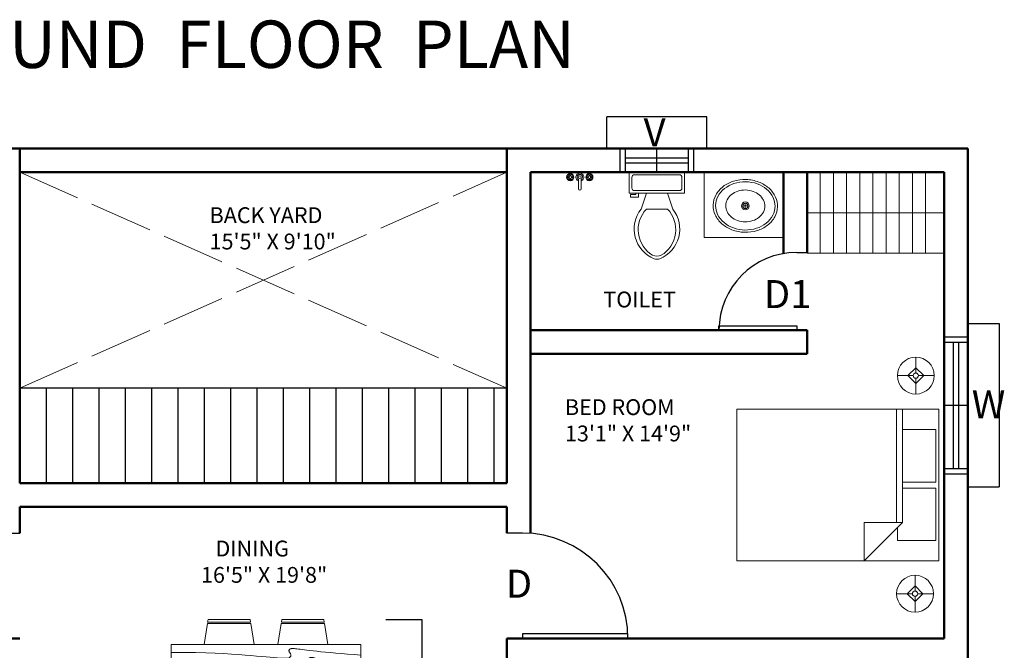
# Model space of a CAD drawing. Units: inches. Extents: x -105 to 1196, y -792 to 119.
# Tile 22 of 23: x 130 to 504, y -121 to 119. Entities that reach past the tile are written whole.
import ezdxf

# ---------------------------------------------------------------- set-up
doc = ezdxf.new("R2010")
doc.units = ezdxf.units.IN
doc.header["$MEASUREMENT"] = 0
doc.linetypes.add('ACAD_ISO02W100', pattern=[15, 12, -3])
for name, color, linetype, lineweight in [('A-ANNO-DIMS', 2, 'Continuous', 18), ('A-ANNO-SYMB', 4, 'ACAD_ISO02W100', 18), ('A-ANNO-TEXT', 7, 'Continuous', 25), ('A-AREA-IDEN', 7, 'Continuous', 25), ('A-DOOR', 4, 'Continuous', 25), ('A-FLOR-FIXT', 8, 'Continuous', 18), ('A-FLOR-STRS', 4, 'Continuous', 25), ('A-FURN', 8, 'Continuous', 18), ('A-GLAZ', 4, 'Continuous', 25), ('A-WALL', 3, 'Continuous', 50)]:
    doc.layers.add(name, color=color, linetype=linetype, lineweight=lineweight)
doc.styles.get("Standard").update_dxf_attribs({"font": 'arial.ttf'})
doc.dimstyles.get("Standard").update_dxf_attribs({"dimtxt": 0.18, "dimasz": 0.18, "dimexe": 0.18, "dimexo": 0.0625, "dimgap": 0.09, "dimtad": 0, "dimtih": 1, "dimtoh": 1, "dimdec": 1, "dimzin": 0, "dimdsep": 46, "dimlunit": 4, "dimtxsty": 'Standard', "dimcen": 0.09, "dimadec": 0, "dimazin": 0, "dimtfac": 1, "dimtdec": 1, "dimtofl": 0, "dimtmove": 0, "dimatfit": 3, "dimfxl": 1, "dimtolj": 1, "dimtzin": 0, "dimarcsym": 0})

# ---------------------------------------------------------------- blocks, each defined once
blk = doc.blocks.new('*U4')
for p, q in [((0, 0), (0, -6)), ((40, 0), (40, -6))]:
    blk.add_line(p, q)
blk.add_lwpolyline([(0, 0), (0, 40), (1.75, 40), (1.75, 0)], close=True)
blk.add_arc((0, 0), 40, 0, 90)
blk = doc.blocks.new('*U5')
for p, q in [((-750, 0), (-750, 100)), ((0, 0), (0, 100))]:
    blk.add_line(p, q)
blk.add_lwpolyline([(0, 0), (0, -750), (-43.75, -750), (-43.75, 0)], close=True)
blk.add_arc((0, 0), 750, 180, 270)
blk = doc.blocks.new('*U6')
for p, q in [((0, 0), (0, 6)), ((40, 0), (40, 6))]:
    blk.add_line(p, q)
blk.add_lwpolyline([(0, 0), (0, -40), (1.75, -40), (1.75, 0)], close=True)
blk.add_arc((0, 0), 40, 270, 0)
blk = doc.blocks.new('Sink - Oval top')
for p, q in [((-1, 0), (1, 0)), ((0, 1), (0, -1))]:
    blk.add_line(p, q)
for points in [[(-12.23, 0.39, 0.117634), (-11.46, -3.36, 0.104469), (-8.88, -6.8, 0.090016), (-5.08, -9.07, 0.08192), (-0.32, -10.02, 0.08192), (4.49, -9.38, 0.090016), (8.42, -7.36, 0.104469), (11.22, -4.09, 0.117634), (12.23, -0.39, 0.117634), (11.46, 3.36, 0.104469), (8.88, 6.8, 0.090016), (5.08, 9.07, 0.08192), (0.32, 10.02, 0.08192), (-4.49, 9.38, 0.090016), (-8.42, 7.36, 0.104469), (-11.22, 4.09, 0.117634)], [(-11.29, 0.16, 0.118622), (-10.52, -3.25, 0.104678), (-8.07, -6.36, 0.089562), (-4.54, -8.37, 0.081185), (-0.13, -9.15, 0.081185), (4.3, -8.49, 0.089562), (7.89, -6.58, 0.104678), (10.42, -3.55, 0.118622), (11.29, -0.16, 0.118622), (10.52, 3.25, 0.104678), (8.07, 6.36, 0.089562), (4.54, 8.37, 0.081185), (0.13, 9.15, 0.081185), (-4.3, 8.49, 0.089562), (-7.89, 6.58, 0.104678), (-10.42, 3.55, 0.118622)], [(-7.42, 0.08, 0.118283), (-6.91, -2.17, 0.104607), (-5.29, -4.21, 0.089718), (-2.97, -5.53, 0.081436), (-0.07, -6.04, 0.081436), (2.84, -5.59, 0.089718), (5.2, -4.33, 0.104607), (6.86, -2.32, 0.118283), (7.42, -0.08, 0.118283), (6.91, 2.17, 0.104607), (5.29, 4.21, 0.089718), (2.97, 5.53, 0.081436), (0.07, 6.04, 0.081436), (-2.84, 5.59, 0.089718), (-5.2, 4.33, 0.104607), (-6.86, 2.32, 0.118283)]]:
    blk.add_lwpolyline(points, format="xyb", close=True)
for radius in [1.5, 1]:
    blk.add_circle((0, 0), radius)
blk = doc.blocks.new('Toilet - top')
for p, q in [((9.5, -6), (9.5, -2)), ((-10, -8.5), (-8, -8.5)), ((-10, -9.5), (-10, -8.5)), ((-7, -9.5), (-10, -9.5)), ((-8, -8.5), (-8, -8)), ((-7, -8), (-7, -9.5)), ((-4, -8), (-6, -14)), ((4, -8), (6, -14)), ((4, -14), (-4, -14))]:
    blk.add_line(p, q)
blk.add_lwpolyline([(10.5, -8), (10.5, 0), (-10.5, 0), (-10.5, -8)], close=True)
for points in [[(-9.5, -2), (-9.5, -6)], [(8.5, -1), (-8.5, -1)], [(-8.5, -7), (8.5, -7)]]:
    blk.add_lwpolyline(points)
for centre, radius, start, end in [((-8.62, -1.88), 0.884, 81.8699, 188.1301), ((8.62, -1.88), 0.884, 351.8699, 98.1301), ((-8.62, -6.12), 0.884, 171.8699, 278.1301), ((8.62, -6.12), 0.884, 261.8699, 8.1301), ((3.52, -21.58), 12.17, 141.4691, 247.9714), ((4.2, -21.82), 11.33, 136.3677, 238.9468), ((-3.52, -21.58), 12.17, 292.0284, 38.5307), ((-4.2, -21.82), 11.33, 301.053, 43.6321), ((0, -27.88), 4, 245.7318, 294.2682), ((0, -29), 4, 254.8605, 285.1395)]:
    blk.add_arc(centre, radius, start, end)
blk = doc.blocks.new('Faucet - Bathroom top')
for p, q in [((-4.107, 0.125), (-4.375, 0.125)), ((-3.75, 0.4788), (-3.75, 0.75)), ((-3.5, 0.482), (-3.5, 0.75)), ((-3.1461, 0.125), (-2.875, 0.125)), ((3.143, 0.125), (2.875, 0.125)), ((3.5, 0.4788), (3.5, 0.75)), ((3.75, 0.482), (3.75, 0.75)), ((4.1039, 0.125), (4.375, 0.125)), ((-4.1039, -0.125), (-4.375, -0.125)), ((-3.75, -0.4821), (-3.75, -0.75)), ((-3.5, -0.4789), (-3.5, -0.75)), ((-3.143, -0.125), (-2.875, -0.125)), ((-0.5, -0.8639), (-0.5, -4.5)), ((0.5, -4.5), (0.5, -0.8631)), ((3.1461, -0.125), (2.875, -0.125)), ((3.5, -0.4821), (3.5, -0.75)), ((3.75, -0.4789), (3.75, -0.75)), ((4.107, -0.125), (4.375, -0.125))]:
    blk.add_line(p, q)
for centre, radius in [((-3.625, 0), 1.375), ((-4.625, 0), 0.2795), ((-3.625, 0), 0.5), ((-3.625, 1), 0.2795), ((-2.625, 0), 0.2795), ((0, 0), 0.5), ((3.625, 0), 1.375), ((2.625, 0), 0.2795), ((3.625, 0), 0.5), ((3.625, 1), 0.2795), ((4.625, 0), 0.2795), ((-3.625, -1), 0.2795), ((3.625, -1), 0.2795)]:
    blk.add_circle(centre, radius)
for centre, radius, start, end in [((-3.625, 0), 1, 105.2407, 164.2093), ((-3.625, 0), 1, 16.44125, 74.07887), ((0, 0), 1.5, 289.6514, 250.3603), ((0, 0), 1, 300.3431, 239.7554), ((3.625, 0), 1, 106.12, 164.0884), ((3.625, 0), 1, 16.23422, 73.90469), ((-3.625, 0), 1, 196.2342, 253.9047), ((-3.625, 0), 1, 286.12, 344.0884), ((3.625, 0), 1, 196.4413, 254.0789), ((3.625, 0), 1, 285.2407, 344.2093), ((0, -4.5), 0.5, 180, 0)]:
    blk.add_arc(centre, radius, start, end)
blk = doc.blocks.new('Bed - Queen')
for p, q in [((0, -80.00003), (0, 0)), ((0, 0), (59.99999, 0)), ((59.99999, 0), (59.99999, -80.00003)), ((7.99999, -1.2), (28.79998, -1.2)), ((7.99999, -14.4), (7.99999, -1.2)), ((28.79998, -1.2), (28.79998, -14.4)), ((31.19999, -1.2), (51.99999, -1.2)), ((31.19999, -14.4), (31.19999, -1.2)), ((51.99999, -1.2), (51.99999, -16.4)), ((0, -14.4), (44.8, -14.4)), ((59.99999, -29.6), (44.8, -14.4)), ((44.8, -14.4), (44.8, -29.6)), ((44.8, -16.8), (0, -16.8)), ((51.99999, -16.4), (46.79936, -16.4)), ((44.8, -29.6), (59.99999, -29.6)), ((59.99999, -80.00003), (0, -80.00003))]:
    blk.add_line(p, q)
blk = doc.blocks.new('Lamp - Table')
for p, q in [((0, 7), (0, 1)), ((-1, 0), (-7, 0)), ((0, 3), (-3, 0)), ((-3, 0), (0, -3)), ((3, 0), (0, 3)), ((0, -3), (3, 0)), ((1, 0), (7, 0)), ((0, -1), (0, -7))]:
    blk.add_line(p, q)
for radius in [7, 1]:
    blk.add_circle((0, 0), radius)
blk = doc.blocks.new('Dining Set - 36 x 72 in.')
for p, q in [((-22, 27.5), (-22.1562, 26.50042)), ((-5.8416, 26.5), (-22.1534, 26.5)), ((-22, 27.5), (-6, 27.5)), ((-5.8437, 26.49966), (-6, 27.5)), ((6, 27.5), (5.8438, 26.50042)), ((22.1584, 26.5), (5.8466, 26.5)), ((6, 27.5), (22, 27.5)), ((22.1563, 26.49966), (22, 27.5)), ((-22.2343, 26.00059), (-23.4847, 17.99762)), ((-22.2304, 26), (-5.7608, 26)), ((-4.5152, 17.99762), (-5.7655, 25.99926)), ((5.7657, 26.00059), (4.5153, 17.99762)), ((5.7696, 26), (22.2392, 26)), ((23.4848, 17.99762), (22.2345, 25.99926)), ((36, 18), (-36, 18)), ((-36, 18), (-36, -18)), ((36, -18), (36, 18)), ((-45.5, 8), (-44.5004, 8.15617)), ((-45.5, 8), (-45.5, -8)), ((-44.5, -8.15843), (-44.5, 8.15338)), ((-44.0006, 8.23428), (-35.9976, 9.48474)), ((-44, 8.23041), (-44, -8.23915)), ((44.0006, 8.23428), (35.9976, 9.48474)), ((44, 8.23041), (44, -8.23915)), ((44.5, -8.15843), (44.5, 8.15338)), ((45.5, 8), (44.5005, 8.15617)), ((45.5, 8), (45.5, -8)), ((-44.4997, -8.15631), (-45.5, -8)), ((-35.9976, -9.48476), (-43.9993, -8.2345)), ((35.9976, -9.48476), (43.9993, -8.2345)), ((44.4997, -8.15631), (45.5, -8)), ((-36, -18), (36, -18)), ((-22.2343, -26.0006), (-23.4847, -17.99762)), ((-4.5152, -17.99762), (-5.7655, -25.99928)), ((5.7657, -26.0006), (4.5153, -17.99762)), ((23.4848, -17.99762), (22.2345, -25.99928)), ((-22.2304, -26), (-5.7608, -26)), ((5.7696, -26), (22.2392, -26)), ((-22, -27.5), (-22.1562, -26.50044)), ((-5.8416, -26.5), (-22.1534, -26.5)), ((-22, -27.5), (-6, -27.5)), ((-5.8437, -26.49967), (-6, -27.5)), ((6, -27.5), (5.8438, -26.50044)), ((22.1584, -26.5), (5.8466, -26.5)), ((6, -27.5), (22, -27.5)), ((22.1563, -26.49967), (22, -27.5))]:
    blk.add_line(p, q)
for points in [[(-36, 15), (-31.1772, 14.97754), (-26.8079, 14.91406), (-22.8538, 14.81543), (-19.276, 14.6875), (-16.0362, 14.53613), (-13.0957, 14.36718), (-10.4159, 14.18652), (-7.9583, 14), (-5.6904, 13.81315), (-3.6035, 13.63021), (-1.6954, 13.45508), (0.0365, 13.29166), (1.5945, 13.14388), (2.9811, 13.01562), (4.1988, 12.9108), (5.25, 12.83333), (6.1393, 12.78613), (6.8802, 12.76823), (7.4883, 12.77767), (7.9792, 12.8125), (8.3685, 12.87077), (8.6719, 12.95052), (8.9049, 13.0498), (9.0833, 13.16666), (9.2205, 13.29899), (9.3216, 13.44401), (9.3895, 13.59879), (9.4271, 13.76041), (9.4373, 13.92594), (9.4232, 14.09245), (9.3875, 14.257), (9.3333, 14.41666), (9.2638, 14.56917), (9.1836, 14.71484), (9.0975, 14.85465), (9.0104, 14.98958), (8.9272, 15.1206), (8.8529, 15.2487), (8.7922, 15.37483), (8.75, 15.5), (8.7305, 15.62467), (8.7344, 15.74739), (8.7617, 15.86621), (8.8125, 15.97916), (8.8867, 16.08431), (8.9844, 16.17968), (9.1055, 16.26334), (9.25, 16.33333), (9.4189, 16.38802), (9.6172, 16.42708), (9.8506, 16.45052), (10.125, 16.45833), (10.4463, 16.45052), (10.8203, 16.42708), (11.2529, 16.38802), (11.75, 16.33333), (12.3184, 16.26318), (12.9694, 16.17838), (13.7151, 16.07991), (14.5677, 15.96875), (15.5395, 15.84586), (16.6426, 15.71224), (17.8893, 15.56884), (19.2917, 15.41666), (20.859, 15.25667), (22.5879, 15.08984), (24.4721, 14.91715), (26.5052, 14.73958), (28.6809, 14.5581), (30.9929, 14.3737), (33.4347, 14.18733), (36, 14)], [(-36, 10), (-28.9766, 10.14274), (-23.1725, 10.20442), (-18.4241, 10.19775), (-14.5677, 10.13541), (-11.4399, 10.03011), (-8.877, 9.89453), (-6.7154, 9.74137), (-4.7917, 9.58333), (-2.9698, 9.43082), (-1.2246, 9.28515), (0.4415, 9.14534), (2.026, 9.01041), (3.5266, 8.87939), (4.9408, 8.7513), (6.266, 8.62516), (7.5, 8.5), (8.6411, 8.37549), (9.6914, 8.2539), (10.6538, 8.13818), (11.5312, 8.03125), (12.3267, 7.93603), (13.043, 7.85547), (13.6831, 7.79248), (14.25, 7.75), (14.7471, 7.7303), (15.1797, 7.73307), (15.5537, 7.75732), (15.875, 7.80208), (16.1494, 7.86637), (16.3828, 7.94922), (16.5811, 8.04964), (16.75, 8.16666), (16.8944, 8.29915), (17.0143, 8.44531), (17.1089, 8.60319), (17.1771, 8.77083), (17.218, 8.94629), (17.2305, 9.1276), (17.2137, 9.31282), (17.1667, 9.5), (17.0895, 9.6875), (16.987, 9.875), (16.8649, 10.0625), (16.7292, 10.25), (16.5856, 10.4375), (16.4401, 10.625), (16.2985, 10.8125), (16.1667, 11), (16.05, 11.18733), (15.9518, 11.3737), (15.8752, 11.5581), (15.8229, 11.73958), (15.798, 11.91715), (15.8034, 12.08984), (15.842, 12.25667), (15.9167, 12.41666), (16.0295, 12.56836), (16.1784, 12.70833), (16.3605, 12.83268), (16.5729, 12.9375), (16.8127, 13.01888), (17.0768, 13.07291), (17.3625, 13.0957), (17.6667, 13.08333), (17.9894, 13.03312), (18.3418, 12.94726), (18.7382, 12.82918), (19.1927, 12.68229), (19.7195, 12.51001), (20.3327, 12.31575), (21.0465, 12.10294), (21.875, 11.875), (22.8357, 11.63354), (23.959, 11.37304), (25.2786, 11.08618), (26.8282, 10.76562), (28.6414, 10.40405), (30.752, 9.99414), (33.1936, 9.52856), (36, 9)], [(-36, 5.5), (-30.7157, 5.3348), (-26.069, 5.20963), (-21.9946, 5.11767), (-18.4271, 5.05208), (-15.3009, 5.00602), (-12.5508, 4.97265), (-10.1112, 4.94515), (-7.9167, 4.91666), (-5.909, 4.88167), (-4.0586, 4.83984), (-2.3429, 4.79215), (-0.7396, 4.73958), (0.7739, 4.6831), (2.22, 4.6237), (3.6213, 4.56233), (5, 4.5), (6.373, 4.43782), (7.7344, 4.3776), (9.0723, 4.32129), (10.375, 4.27083), (11.6309, 4.22819), (12.8281, 4.19531), (13.9551, 4.17415), (15, 4.16666), (15.954, 4.17448), (16.819, 4.19791), (17.6001, 4.23698), (18.3021, 4.29166), (18.9299, 4.36198), (19.4883, 4.44791), (19.9823, 4.54948), (20.4167, 4.66666), (20.7969, 4.79899), (21.1302, 4.94401), (21.4245, 5.09879), (21.6875, 5.26041), (21.9271, 5.42594), (22.1511, 5.59245), (22.3672, 5.757), (22.5834, 5.91666), (22.8065, 6.06868), (23.0404, 6.21093), (23.2879, 6.34147), (23.5521, 6.45833), (23.8358, 6.55957), (24.142, 6.64323), (24.4735, 6.70735), (24.8334, 6.75), (25.2235, 6.76969), (25.642, 6.76692), (26.0858, 6.74267), (26.5521, 6.69791), (27.0379, 6.63362), (27.5404, 6.55078), (28.0565, 6.45036), (28.5834, 6.33333), (29.1242, 6.19987), (29.7071, 6.04687), (30.3661, 5.87044), (31.1354, 5.66666), (32.0493, 5.43164), (33.142, 5.16146), (34.4475, 4.85221), (36, 4.5)], [(-36, -1), (-30.7915, -0.6591), (-26.0195, -0.38216), (-21.6519, -0.16284), (-17.6563, 0.00521), (-14.0005, 0.12833), (-10.6523, 0.21289), (-7.5796, 0.26522), (-4.75, 0.29166), (-2.134, 0.29793), (0.2878, 0.28711), (2.5317, 0.26163), (4.6146, 0.22396), (6.5529, 0.17651), (8.3633, 0.12174), (10.0623, 0.06209), (11.6667, 0), (13.1899, -0.06201), (14.6341, -0.1211), (15.9982, -0.17432), (17.2813, -0.21875), (18.4823, -0.25147), (19.6003, -0.26953), (20.6343, -0.27002), (21.5834, -0.25), (22.4481, -0.20768), (23.2357, -0.14584), (23.9549, -0.06836), (24.6146, 0.02083), (25.2235, 0.11784), (25.7904, 0.21875), (26.3241, 0.31966), (26.8334, 0.41666), (27.3265, 0.50618), (27.8099, 0.58593), (28.2894, 0.65397), (28.7709, 0.70833), (29.2601, 0.74707), (29.763, 0.76823), (30.2855, 0.76985), (30.8334, 0.75), (31.4088, 0.70784), (31.9994, 0.64713), (32.589, 0.57275), (33.1615, 0.48958), (33.7008, 0.4025), (34.1908, 0.3164), (34.6153, 0.23616), (34.9584, 0.16666), (35.2099, 0.11165), (35.3848, 0.07031), (35.504, 0.04069), (35.5886, 0.02083), (35.6594, 0.00879), (35.7377, 0.0026), (35.8442, 0.00032), (36, 0)], [(-36, -6.5), (-27.1843, -6.31267), (-20.084, -6.1263), (-14.469, -5.9419), (-10.1094, -5.76042), (-6.7752, -5.58285), (-4.2363, -5.41016), (-2.2629, -5.24333), (-0.625, -5.08334), (0.8708, -4.93099), (2.2715, -4.78646), (3.5872, -4.64974), (4.8281, -4.52084), (6.0046, -4.39974), (7.127, -4.28646), (8.2053, -4.18099), (9.25, -4.08334), (10.2705, -3.99382), (11.2734, -3.91407), (12.2647, -3.84603), (13.25, -3.79167), (14.2354, -3.75293), (15.2266, -3.73177), (16.2295, -3.73015), (17.25, -3.75), (18.2912, -3.79248), (19.3451, -3.85547), (20.4009, -3.93604), (21.4479, -4.03125), (22.4754, -4.13819), (23.4727, -4.25391), (24.4289, -4.37549), (25.3334, -4.5), (26.1785, -4.62492), (26.9694, -4.74935), (27.7145, -4.87281), (28.4219, -4.99479), (29.1, -5.11483), (29.7572, -5.23242), (30.4016, -5.34709), (31.0417, -5.45834), (31.6837, -5.56437), (32.3262, -5.65821), (32.9658, -5.73153), (33.599, -5.77604), (34.2224, -5.78345), (34.8327, -5.74545), (35.4264, -5.65373), (36, -5.5)], [(-36, -10), (-26.4022, -9.81299), (-18.4675, -9.62891), (-11.9839, -9.45069), (-6.7396, -9.28125), (-2.5226, -9.12354), (0.8789, -8.98047), (3.6769, -8.85498), (6.0833, -8.75), (8.2767, -8.66765), (10.3021, -8.60677), (12.1712, -8.56543), (13.8958, -8.54167), (15.4876, -8.53353), (16.9583, -8.53907), (18.3197, -8.55632), (19.5834, -8.58334), (20.7616, -8.61841), (21.8685, -8.66081), (22.9188, -8.71004), (23.9271, -8.76563), (24.9081, -8.82707), (25.8763, -8.89388), (26.8465, -8.96558), (27.8334, -9.04167), (28.8474, -9.12118), (29.8828, -9.20117), (30.93, -9.27824), (31.9792, -9.34896), (33.0205, -9.40991), (34.0443, -9.45768), (35.0407, -9.48885), (36, -9.5)], [(-36, -14.5), (-30.0881, -14.33513), (-25.0332, -14.21224), (-20.7312, -14.12647), (-17.0781, -14.07292), (-13.97, -14.04671), (-11.3027, -14.04297), (-8.9724, -14.05681), (-6.875, -14.08334), (-4.9224, -14.11833), (-3.0905, -14.16016), (-1.3709, -14.20785), (0.2448, -14.26042), (1.7647, -14.3169), (3.1973, -14.3763), (4.5507, -14.43767), (5.8333, -14.5), (7.0554, -14.5621), (8.235, -14.62175), (9.3922, -14.67652), (10.5469, -14.72396), (11.7192, -14.76164), (12.929, -14.78711), (14.1965, -14.79794), (15.5417, -14.79167), (16.9933, -14.76424), (18.6152, -14.70508), (20.4804, -14.60197), (22.6615, -14.44271), (25.2312, -14.21509), (28.2624, -13.9069), (31.8277, -13.50594), (36, -13)]]:
    blk.add_lwpolyline(points)
blk = doc.blocks.new('WIN-1200')
at = {"ltscale": 2}
for p, q in [((12, 62), (0, 62)), ((0, 0), (0, 62)), ((12, 57), (12, 62)), ((12, 5), (12, 0)), ((12, 0), (0, 0))]:
    blk.add_line(p, q, dxfattribs=at)
for p, q in [((21, 57), (12, 57)), ((21, 5), (12, 5))]:
    blk.add_line(p, q)
blk = doc.blocks.new('VENT-600')
for p, q in [((0, 9), (0, 21)), ((38, 21), (0, 21)), ((38, 9), (38, 21)), ((5, 9), (0, 9)), ((5, 0), (5, 9)), ((33, 0), (33, 9)), ((33, 9), (38, 9))]:
    blk.add_line(p, q)
blk = doc.blocks.new('*D76')
at = {"layer": 'A-ANNO-DIMS', "color": 0, "lineweight": -2, "transparency": 16777216}
for p, q in [((268.83, -109.03), (282.6, -109.03)), ((282.42, -109.21), (282.42, -136.35)), ((282.42, -163.85), (282.42, -136.71)), ((268.83, -164.03), (282.6, -164.03))]:
    blk.add_line(p, q, dxfattribs=at)
at = {"layer": 'A-ANNO-DIMS', "color": 0, "transparency": 16777216}
for points in [[(282.39, -109.21), (282.45, -109.21), (282.42, -109.03)], [(282.39, -163.85), (282.45, -163.85), (282.42, -164.03)]]:
    blk.add_solid(points, dxfattribs=at)
at = {"layer": 'Defpoints', "color": 0, "transparency": 16777216}
for p in [(268.77, -109.03), (282.42, -109.03), (268.77, -164.03)]:
    blk.add_point(p, dxfattribs=at)
at = {"layer": 'A-ANNO-DIMS', "color": 0, "transparency": 16777216, "insert": (282.42, -136.53), "char_height": 0.18, "attachment_point": 5}
blk.add_mtext('\\A1;4\'-7"', dxfattribs=at)

msp = doc.modelspace()

# ---------------------------------------------------------------- linework, layer by layer
at = {"layer": 'A-ANNO-SYMB', "ltscale": 2}
for p, q in [((129.74, -21.23), (314.74, 60.77)), ((129.74, 60.77), (314.74, -21.23))]:
    msp.add_line(p, q, dxfattribs=at)
at = {"layer": 'A-FLOR-FIXT'}
for p, q in [((389.61, 35.96), (389.61, 60.77)), ((433.74, 30.04), (433.74, 60.77)), ((438.74, 30.04), (438.74, 60.77)), ((443.74, 30.04), (443.74, 60.77)), ((448.74, 30.04), (448.74, 60.77)), ((453.74, 30.04), (453.74, 60.77)), ((458.74, 30.04), (458.74, 60.77)), ((463.74, 30.04), (463.74, 60.77)), ((468.74, 30.04), (468.74, 60.77)), ((473.74, 30.04), (473.74, 60.77)), ((428.74, 45.4), (480.74, 45.4)), ((419.74, 35.96), (389.61, 35.96)), ((428.74, 30.04), (480.74, 30.04))]:
    msp.add_line(p, q, dxfattribs=at)
at = {"layer": 'A-FLOR-STRS'}
for p, q in [((314.74, -21.23), (129.74, -21.23)), ((139.74, -21.23), (139.74, -57.23)), ((149.74, -21.23), (149.74, -57.23)), ((159.74, -21.23), (159.74, -57.23)), ((169.74, -21.23), (169.74, -57.23)), ((179.74, -21.23), (179.74, -57.23)), ((189.74, -21.23), (189.74, -57.23)), ((199.74, -21.23), (199.74, -57.23)), ((209.74, -21.23), (209.74, -57.23)), ((219.74, -21.23), (219.74, -57.23)), ((229.74, -21.23), (229.74, -57.23)), ((239.74, -21.23), (239.74, -57.23)), ((249.74, -21.23), (249.74, -57.23)), ((259.74, -21.23), (259.74, -57.23)), ((269.74, -21.23), (269.74, -57.23)), ((279.74, -21.23), (279.74, -57.23)), ((289.74, -21.23), (289.74, -57.23)), ((299.74, -21.23), (299.74, -57.23)), ((309.74, -21.23), (309.74, -57.23))]:
    msp.add_line(p, q, dxfattribs=at)
at = {"layer": 'A-GLAZ'}
for p, q in [((359.74, 60.77), (359.74, 69.77)), ((371.74, 60.77), (371.74, 69.77)), ((383.74, 60.77), (383.74, 69.77)), ((359.74, 66.27), (383.74, 66.27)), ((359.74, 64.27), (383.74, 64.27)), ((480.74, -3.73), (489.74, -3.73)), ((484.24, -3.73), (484.24, -51.73)), ((486.24, -3.73), (486.24, -51.73)), ((480.74, -27.73), (489.74, -27.73)), ((480.74, -51.73), (489.74, -51.73))]:
    msp.add_line(p, q, dxfattribs=at)
at = {"layer": 'A-WALL'}
for p, q in [((-45.26, 69.77), (129.74, 69.77)), ((129.74, 69.77), (129.74, -57.23)), ((314.74, 69.77), (489.74, 69.77)), ((314.74, 69.77), (314.74, -57.23)), ((489.74, 69.77), (489.74, -125.23)), ((314.74, 60.77), (314.74, -57.23)), ((323.74, 60.77), (323.74, -76.34)), ((323.74, 60.77), (323.74, 0.77)), ((323.74, 60.77), (480.74, 60.77)), ((419.74, 29.86), (419.74, 60.77)), ((428.74, 30.04), (428.74, 60.77)), ((480.74, 60.77), (480.74, -116.23)), ((323.74, 0.77), (428.74, 0.77)), ((428.74, -8.23), (428.74, 0.77)), ((323.74, -8.23), (428.74, -8.23)), ((314.74, -57.23), (129.74, -57.23)), ((314.74, -66.23), (129.74, -66.23)), ((129.74, -66.23), (129.74, -76.23)), ((314.74, -66.23), (314.74, -76.23)), ((-36.26, -116.23), (129.74, -116.23)), ((480.74, -116.23), (314.74, -116.23)), ((314.74, -116.23), (314.74, -228.23))]:
    msp.add_line(p, q, dxfattribs=at)
at = {"layer": 'A-WALL', "ltscale": 3}
for p, q in [((129.74, 69.77), (323.74, 69.77)), ((129.74, 60.77), (314.74, 60.77))]:
    msp.add_line(p, q, dxfattribs=at)

# ---------------------------------------------------------------- block references
at = {"layer": 'A-DOOR', "xscale": 0.0393700787401575, "yscale": 0.0393700787401575, "zscale": 0.0393700787401575, "rotation": 270}
msp.add_blockref('*U5', (424.81, 0.77), dxfattribs=at)
at = {"layer": 'A-DOOR', "rotation": 90}
for name, p in [('*U4', (123.74, -116.23)), ('*U6', (320.74, -116.23))]:
    msp.add_blockref(name, p, dxfattribs=at)
at = {"layer": 'A-FLOR-FIXT'}
for name, p in [('Faucet - Bathroom top', (342.45, 58.89)), ('Toilet - top', (371.74, 60.77)), ('Sink - Oval top', (405.29, 47.97))]:
    msp.add_blockref(name, p, dxfattribs=at)
at = {"layer": 'A-FURN'}
for name, p in [('Lamp - Table', (470.03, -16.46)), ('Lamp - Table', (469.74, -99.24)), ('Dining Set - 36 x 72 in.', (223.27, -136.53))]:
    msp.add_blockref(name, p, dxfattribs=at)
at = {"layer": 'A-FURN', "xscale": 0.9593862173514477, "yscale": 0.9593862173514477, "zscale": 0.9593862173514477, "rotation": 270}
msp.add_blockref('Bed - Queen', (478.82, -29.22), dxfattribs=at)
at = {"layer": 'A-GLAZ'}
msp.add_blockref('VENT-600', (352.74, 60.77), dxfattribs=at)
at = {"layer": 'A-GLAZ', "rotation": 180}
msp.add_blockref('WIN-1200', (501.74, 3.27), dxfattribs=at)

# ---------------------------------------------------------------- texts
at = {"layer": 'A-ANNO-TEXT'}
for s, height, p in [('GROUND  FLOOR  PLAN', 18, (75.01, 100.34)), ('V', 10.64, (366.67, 70.59)), ('D1', 10.636, (412.34, 9.17)), ('W', 10.64, (491.29, -32.72)), ('D', 10.64, (314.35, -100.77))]:
    msp.add_text(s, height=height, dxfattribs=at).set_placement(p)
at = {"layer": 'A-AREA-IDEN', "char_height": 6, "attachment_point": 1}
for s, insert in [('BACK YARD\\P15\'5" X 9\'10"', (201.86, 47.45)), ('TOILET', (351.37, 15.44)), ('BED ROOM\\P13\'1" X 14\'9"', (336.81, -25.42)), ('   DINING \\P16\'5" X 19\'8"', (198.59, -79.1))]:
    msp.add_mtext_dynamic_manual_height_columns(s, width=59.5623, gutter_width=1, heights=[0], dxfattribs=dict(at, insert=insert))

# ---------------------------------------------------------------- dimensions: what is measured, and where the dimension line sits
at = {"layer": 'A-ANNO-DIMS'}
dim = msp.add_linear_dim(base=(282.42, -109.03), p1=(268.77, -164.03), p2=(268.77, -109.03), angle=90, dimstyle='Standard', override={"dimdec": 1, "dimlfac": 1, "dimrnd": 0, "dimzin": 1, "dimdsep": 46, "dimlunit": 4, "dimfrac": 2}, dxfattribs=at)
dim.commit()
dim.dimension.update_dxf_attribs({"geometry": '*D76', "text_midpoint": (282.42, -136.53)})

doc.saveas('drawing.dxf')
